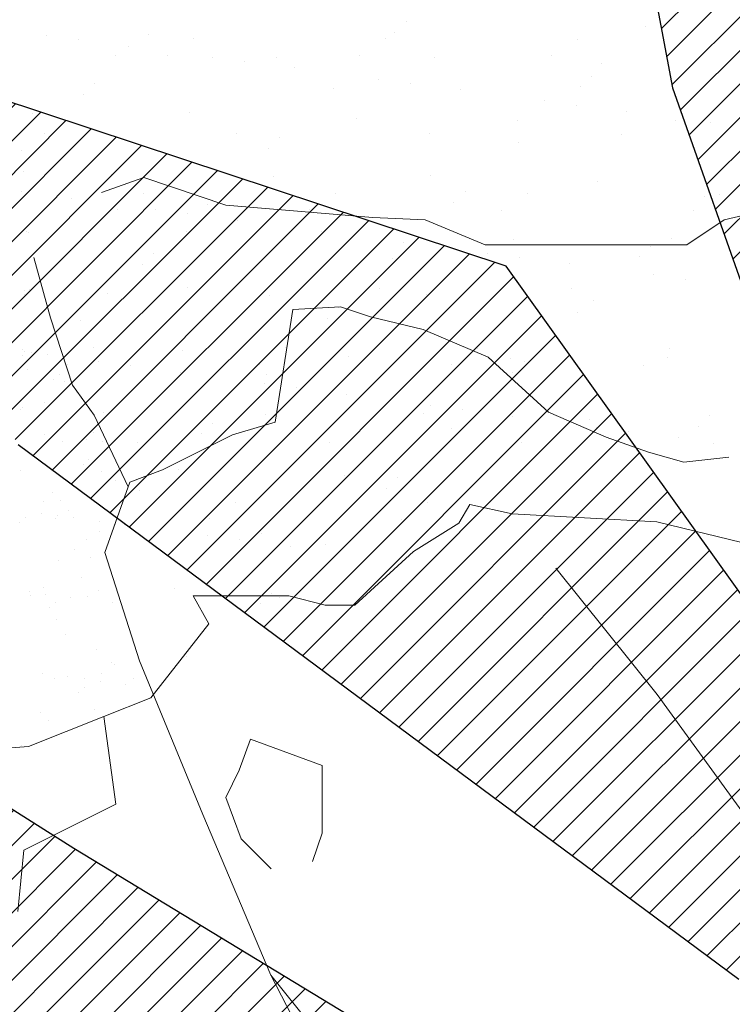
# Model space of a CAD drawing. Units: inches. Extents: x 1986 to 21484, y -1816 to 2016.
# Tile 23 of 85: x 2162.297 to 2166.915, y 1891.95 to 1898.331. Entities that reach past the tile are written whole.
import ezdxf

# ---------------------------------------------------------------- set-up
doc = ezdxf.new("R2010")
doc.units = ezdxf.units.IN
doc.layers.add('L-PLNT', color=84, linetype='Continuous', lineweight=13)
doc.layers.add('vfolhas', color=114, linetype='Continuous', lineweight=5)
doc.layers.add('vfolha2', color=110, linetype='Continuous')
doc.layers.add('vfolhas2', color=102, linetype='Continuous')
pattern_1 = [(45, (-2446.5133113, 50.986076), (-0.004419417382, 0.004419417382), [])]

# ---------------------------------------------------------------- blocks, each defined once
blk = doc.blocks.new('arbusto_PB_verde_grande')
at = {"layer": 'vfolha2'}
h = blk.add_hatch(dxfattribs=at)
h.set_pattern_fill('ANSI31', color=256, scale=0.05, style=0)
h.set_pattern_definition(pattern_1)
h.paths.add_polyline_path([(-0.18963, 0.29704), (-0.08553, 0.20192), (-0.10785, 0.25007), (-0.13202, 0.31865), (-0.25096, 0.48479), (-0.44952, 0.5505), (-0.37946, 0.43789)])
h.paths.add_polyline_path([(0.07911, -0.4071), (0.08214, -0.50631), (0.17255, -0.6355), (0.18428, -0.44151), (0.14904, -0.29177), (0.02625, -0.03934), (0.03527, -0.25376)])
at = {"layer": 'vfolhas'}
h = blk.add_hatch(dxfattribs=at)
h.set_pattern_fill('ANSI31', color=256, scale=0.05, style=0)
h.set_pattern_definition(pattern_1)
h.paths.add_polyline_path([(-0.07279, 0.50669), (-0.18085, 0.65063), (-0.2334, 0.67253), (-0.20712, 0.53176), (-0.10785, 0.25007), (0.02625, -0.03934), (0.00028, 0.09048), (0.00816, 0.16241), (-0.04939, 0.29079)])
h.paths.add_polyline_path([(0.09902, 0.41929), (0.09372, 0.26573), (0.07906, 0.18814), (0.15506, 0.36901), (0.26606, 0.5505), (0.28356, 0.63504), (0.2485, 0.68819), (0.25145, 0.63504), (0.20178, 0.54426)])
h.paths.add_polyline_path([(0.12295, 0.24073), (0.047, 0.06233), (0.02625, -0.03934), (0.11122, 0.04358), (0.18428, 0.09364), (0.27478, 0.19376), (0.3215, 0.25323), (0.44129, 0.38467), (0.47634, 0.57866), (0.41789, 0.45347), (0.28939, 0.30954)])
h.paths.add_polyline_path([(0.58145, -0.03779), (0.70707, 0.01536), (0.78591, 0.04667), (0.74796, 0.06549), (0.62818, 0.08423), (0.52595, 0.09048), (0.39745, 0.04358), (0.02625, -0.03934), (0.25728, -0.03154), (0.43834, -0.0347)])
h.paths.add_polyline_path([(0.52022, -0.03647), (0.43834, -0.0347), (0.25728, -0.03154), (0.02625, -0.03934), (0.17964, -0.08515), (0.53768, -0.13167), (0.69541, -0.15357), (0.78591, -0.07852), (0.70413, -0.10042)])
h.paths.add_polyline_path([(0.27189, -0.21929), (0.14922, -0.14107), (0.02625, -0.03934), (0.15794, -0.31007), (0.29522, -0.42585), (0.41789, -0.49157), (0.56396, -0.56669), (0.5114, -0.48532), (0.39456, -0.34139)])
h.paths.add_polyline_path([(-0.05818, -0.47591), (-0.02312, -0.61984), (0.047, -0.80134), (0.08494, -0.59794), (0.07911, -0.4071), (0.03527, -0.25376), (0.02625, -0.03934), (-0.03773, -0.26001)])
h.paths.add_polyline_path([(-0.24218, 0.14054), (-0.11073, 0.06858), (0.02625, -0.03934), (-0.04235, 0.10871), (-0.21007, 0.23757), (-0.36485, 0.33145), (-0.47874, 0.40341), (-0.54303, 0.46288), (-0.49041, 0.33145), (-0.39408, 0.22192)])
at = {"layer": 'vfolha2'}
for p, q in [((-0.25096, 0.48479), (-0.44952, 0.5505)), ((-0.13202, 0.31865), (-0.25096, 0.48479)), ((-0.37946, 0.43789), (-0.18963, 0.29704))]:
    blk.add_line(p, q, dxfattribs=at)
at = {"layer": 'vfolhas2'}
for p, q in [((-0.2334, 0.67253), (-0.20712, 0.53176)), ((-0.20712, 0.53176), (-0.10785, 0.25007)), ((-0.36485, 0.33145), (-0.47874, 0.40341)), ((-0.21007, 0.23757), (-0.36485, 0.33145))]:
    blk.add_line(p, q, dxfattribs=at)
blk = doc.blocks.new('PLANT-SHRUB')
for p, q in [((2164.8017, 1898.3163), (2164.8017, 1898.3163)), ((2162.47, 1898.2297), (2162.47, 1898.2297)), ((2163.1287, 1898.235), (2163.1287, 1898.235)), ((2164.728, 1898.2488), (2164.728, 1898.2488)), ((2166.3509, 1898.2841), (2166.3509, 1898.2841)), ((2162.678, 1898.2023), (2162.678, 1898.2023)), ((2163.0029, 1898.1596), (2163.0029, 1898.1596)), ((2163.421, 1898.2083), (2163.421, 1898.2083)), ((2164.6656, 1898.206), (2164.6656, 1898.206)), ((2165.9103, 1898.2038), (2165.9103, 1898.2038)), ((2162.9177, 1898.0971), (2162.9177, 1898.0971)), ((2163.2525, 1898.1009), (2163.2525, 1898.1009)), ((2164.4971, 1898.0987), (2164.4971, 1898.0987)), ((2165.7417, 1898.0964), (2165.7417, 1898.0964)), ((2163.5458, 1898.0881), (2163.5458, 1898.0881)), ((2163.7538, 1898.0607), (2163.7538, 1898.0607)), ((2163.9638, 1898.0837), (2163.9638, 1898.0837)), ((2164.9862, 1898.0886), (2164.9862, 1898.0886)), ((2166.0657, 1898.0497), (2166.0657, 1898.0497)), ((2164.0787, 1898.0179), (2164.0787, 1898.0179)), ((2162.781, 1897.9164), (2162.781, 1897.9164)), ((2164.6216, 1897.9464), (2164.6216, 1897.9464)), ((2164.8296, 1897.9191), (2164.8296, 1897.9191)), ((2166.0031, 1897.9655), (2166.0031, 1897.9655)), ((2162.7074, 1897.8489), (2162.7074, 1897.8489)), ((2164.3302, 1897.8842), (2164.3302, 1897.8842)), ((2165.1546, 1897.8763), (2165.1546, 1897.8763)), ((2165.9295, 1897.898), (2165.9295, 1897.898)), ((2165.6974, 1897.8048), (2165.6974, 1897.8048)), ((2165.9055, 1897.7774), (2165.9055, 1897.7774)), ((2162.3772, 1897.7223), (2162.3772, 1897.7223)), ((2163.3996, 1897.7273), (2163.3996, 1897.7273)), ((2166.2304, 1897.7346), (2166.2304, 1897.7346)), ((2164.4791, 1897.6884), (2164.4791, 1897.6884)), ((2165.5253, 1897.675), (2165.5253, 1897.675)), ((2166.5477, 1897.6799), (2166.5477, 1897.6799)), ((2166.7733, 1897.6632), (2166.7733, 1897.6632)), ((2162.4603, 1897.5963), (2162.4603, 1897.5963)), ((2163.705, 1897.594), (2163.705, 1897.594)), ((2164.9496, 1897.5918), (2164.9496, 1897.5918)), ((2166.1942, 1897.5895), (2166.1942, 1897.5895)), ((2163.9825, 1897.5656), (2163.9825, 1897.5656)), ((2165.5317, 1897.5335), (2165.5317, 1897.5335)), ((2162.3096, 1897.4844), (2162.3096, 1897.4844)), ((2162.3096, 1897.4844), (2162.3096, 1897.4844)), ((2163.9088, 1897.4981), (2163.9088, 1897.4981)), ((2162.3185, 1897.3493), (2162.3185, 1897.3493)), ((2163.1007, 1897.3074), (2162.8262, 1897.2106)), ((2162.8925, 1897.327), (2162.8925, 1897.327)), ((2163.6336, 1897.1299), (2163.1007, 1897.3074)), ((2163.9387, 1897.3136), (2163.9387, 1897.3136)), ((2164.9611, 1897.3185), (2164.9611, 1897.3185)), ((2166.0405, 1897.2796), (2166.0405, 1897.2796)), ((2162.3095, 1897.216), (2162.3095, 1897.216)), ((2162.3095, 1897.216), (2162.3095, 1897.216)), ((2162.3095, 1897.216), (2162.3095, 1897.216)), ((2163.0982, 1897.2075), (2163.0982, 1897.2075)), ((2164.3428, 1897.2052), (2164.3428, 1897.2052)), ((2165.184, 1897.2148), (2165.184, 1897.2148)), ((2165.5875, 1897.203), (2165.5875, 1897.203)), ((2166.8321, 1897.2007), (2166.8321, 1897.2007)), ((2162.6344, 1897.1733), (2162.6344, 1897.1733)), ((2165.1103, 1897.1473), (2165.1103, 1897.1473)), ((2166.7331, 1897.1827), (2166.7331, 1897.1827)), ((2162.9297, 1897.1001), (2162.9297, 1897.1001)), ((2163.1773, 1897.1018), (2163.1773, 1897.1018)), ((2163.3853, 1897.0744), (2163.3853, 1897.0744)), ((2163.511, 1897.1336), (2163.511, 1897.1336)), ((2164.5862, 1897.0492), (2163.6336, 1897.1299)), ((2164.1743, 1897.0979), (2164.1743, 1897.0979)), ((2165.4189, 1897.0956), (2165.4189, 1897.0956)), ((2166.6636, 1897.0933), (2166.6636, 1897.0933)), ((2167.202, 1897.1138), (2166.8629, 1897.0331)), ((2163.7102, 1897.0316), (2163.7102, 1897.0316)), ((2164.9253, 1897.0331), (2164.5862, 1897.0492)), ((2165.3128, 1896.8718), (2164.9253, 1897.0331)), ((2166.8629, 1897.0331), (2166.6207, 1896.8718)), ((2162.3402, 1896.9614), (2162.3402, 1896.9614)), ((2162.3521, 1896.9523), (2162.3521, 1896.9523)), ((2162.3521, 1896.9523), (2162.3521, 1896.9523)), ((2163.3745, 1896.9572), (2163.3745, 1896.9572)), ((2164.2531, 1896.9602), (2164.2531, 1896.9602)), ((2164.4539, 1896.9183), (2164.4539, 1896.9183)), ((2164.4611, 1896.9328), (2164.4611, 1896.9328)), ((2164.7861, 1896.89), (2164.7861, 1896.89)), ((2165.5001, 1896.9049), (2165.5001, 1896.9049)), ((2166.5225, 1896.9098), (2166.5225, 1896.9098)), ((2165.3128, 1896.8718), (2165.3128, 1896.8718)), ((2165.8457, 1896.8718), (2165.3128, 1896.8718)), ((2165.3289, 1896.8185), (2165.3289, 1896.8185)), ((2166.2655, 1896.8718), (2165.8457, 1896.8718)), ((2166.6207, 1896.8718), (2166.2655, 1896.8718)), ((2166.3854, 1896.8641), (2166.3854, 1896.8641)), ((2162.4964, 1896.3984), (2162.3874, 1896.7903)), ((2163.1633, 1896.815), (2163.1633, 1896.815)), ((2164.7125, 1896.7828), (2164.7125, 1896.7828)), ((2165.537, 1896.7911), (2165.537, 1896.7911)), ((2166.3118, 1896.7966), (2166.3118, 1896.7966)), ((2163.0897, 1896.7475), (2163.0897, 1896.7475)), ((2165.8619, 1896.7484), (2165.8619, 1896.7484)), ((2166.4048, 1896.6769), (2166.4048, 1896.6769)), ((2166.6128, 1896.6495), (2166.6128, 1896.6495)), ((2162.3276, 1896.5763), (2162.3276, 1896.5763)), ((2162.362, 1896.5813), (2162.362, 1896.5813)), ((2162.3918, 1896.6008), (2162.3918, 1896.6008)), ((2163.3822, 1896.5932), (2163.3822, 1896.5932)), ((2164.6268, 1896.5909), (2164.6268, 1896.5909)), ((2165.8714, 1896.5887), (2165.8714, 1896.5887)), ((2162.3251, 1896.5476), (2162.3251, 1896.5476)), ((2162.8673, 1896.5569), (2162.8673, 1896.5569)), ((2163.9135, 1896.5435), (2163.9135, 1896.5435)), ((2164.9359, 1896.5484), (2164.9359, 1896.5484)), ((2166.0154, 1896.5096), (2166.0154, 1896.5096)), ((2163.9528, 1895.7227), (2164.0665, 1896.4531)), ((2164.0665, 1896.4531), (2164.3751, 1896.4694)), ((2164.0665, 1896.4531), (2164.0665, 1896.4531)), ((2164.3648, 1896.4642), (2164.3648, 1896.4642)), ((2164.3751, 1896.4694), (2164.5701, 1896.4044)), ((2164.3751, 1896.4694), (2164.3751, 1896.4694)), ((2162.638, 1895.9629), (2162.4964, 1896.3984)), ((2162.6919, 1896.383), (2162.6919, 1896.383)), ((2164.2911, 1896.3967), (2164.2911, 1896.3967)), ((2164.5701, 1896.4044), (2164.9112, 1896.3233)), ((2165.914, 1896.432), (2165.914, 1896.432)), ((2164.9112, 1896.3233), (2165.3335, 1896.1447)), ((2162.315, 1896.1913), (2162.315, 1896.1913)), ((2162.3269, 1896.1822), (2162.3269, 1896.1822)), ((2162.3269, 1896.1822), (2162.3269, 1896.1822)), ((2162.7754, 1896.2067), (2162.7754, 1896.2067)), ((2163.3493, 1896.1871), (2163.3493, 1896.1871)), ((2164.0201, 1896.2044), (2164.0201, 1896.2044)), ((2165.2647, 1896.2022), (2165.2647, 1896.2022)), ((2166.5093, 1896.1999), (2166.5093, 1896.1999)), ((2162.3146, 1896.1541), (2162.3146, 1896.1541)), ((2162.3749, 1896.1726), (2162.3749, 1896.1726)), ((2162.4789, 1896.1589), (2162.4789, 1896.1589)), ((2164.4287, 1896.1482), (2164.4287, 1896.1482)), ((2165.3335, 1896.1447), (2165.7234, 1895.7876)), ((2165.3335, 1896.1447), (2165.3335, 1896.1447)), ((2165.4749, 1896.1348), (2165.4749, 1896.1348)), ((2166.4973, 1896.1397), (2166.4973, 1896.1397)), ((2162.3441, 1896.0644), (2162.3441, 1896.0644)), ((2162.3441, 1896.0644), (2162.3441, 1896.0644)), ((2162.6069, 1896.0993), (2162.6069, 1896.0993)), ((2162.8088, 1896.1155), (2162.8088, 1896.1155)), ((2163.0168, 1896.0881), (2163.0168, 1896.0881)), ((2163.8515, 1896.097), (2163.8515, 1896.097)), ((2165.0962, 1896.0948), (2165.0962, 1896.0948)), ((2165.5662, 1896.1134), (2165.5662, 1896.1134)), ((2166.3408, 1896.0925), (2166.3408, 1896.0925)), ((2162.5163, 1895.9968), (2162.5163, 1895.9968)), ((2162.5531, 1896.0306), (2162.5531, 1896.0306)), ((2163.3417, 1896.0453), (2163.3417, 1896.0453)), ((2163.8933, 1896.0322), (2163.8933, 1896.0322)), ((2165.4926, 1896.0459), (2165.4926, 1896.0459)), ((2162.5845, 1895.9845), (2162.5845, 1895.9845)), ((2162.7797, 1895.7669), (2162.638, 1895.9629)), ((2163.8846, 1895.9739), (2163.8846, 1895.9739)), ((2164.0926, 1895.9465), (2164.0926, 1895.9465)), ((2164.4176, 1895.9037), (2164.4176, 1895.9037)), ((2162.3024, 1895.8062), (2162.3024, 1895.8062)), ((2162.3174, 1895.8146), (2162.3174, 1895.8146)), ((2162.4566, 1895.847), (2162.4566, 1895.847)), ((2164.9604, 1895.8322), (2164.9604, 1895.8322)), ((2165.1685, 1895.8048), (2165.1685, 1895.8048)), ((2162.9997, 1895.3027), (2162.7797, 1895.7669)), ((2162.8421, 1895.7868), (2162.8421, 1895.7868)), ((2163.8883, 1895.7734), (2163.8883, 1895.7734)), ((2164.9107, 1895.7783), (2164.9107, 1895.7783)), ((2165.4934, 1895.7621), (2165.4934, 1895.7621)), ((2165.7234, 1895.7876), (2166.097, 1895.6253)), ((2165.7234, 1895.7876), (2165.7234, 1895.7876)), ((2165.9902, 1895.7395), (2165.9902, 1895.7395)), ((2166.7677, 1895.7626), (2166.7677, 1895.7626)), ((2163.5456, 1895.7136), (2163.5456, 1895.7136)), ((2163.6766, 1895.6415), (2163.9528, 1895.7227)), ((2165.0948, 1895.6814), (2165.0948, 1895.6814)), ((2166.0363, 1895.6906), (2166.0363, 1895.6906)), ((2166.694, 1895.6951), (2166.694, 1895.6951)), ((2162.4571, 1895.6444), (2162.4571, 1895.6444)), ((2162.7286, 1895.6086), (2162.7286, 1895.6086)), ((2162.7756, 1895.6526), (2162.7756, 1895.6526)), ((2163.2218, 1895.4143), (2163.6766, 1895.6415)), ((2163.4719, 1895.6461), (2163.4719, 1895.6461)), ((2166.097, 1895.6253), (2166.3732, 1895.5279)), ((2166.2443, 1895.6632), (2166.2443, 1895.6632)), ((2166.5692, 1895.6204), (2166.5692, 1895.6204)), ((2162.5719, 1895.5994), (2162.5719, 1895.5994)), ((2162.6913, 1895.5989), (2162.6913, 1895.5989)), ((2162.8326, 1895.595), (2162.8326, 1895.595)), ((2163.0594, 1895.5924), (2163.0594, 1895.5924)), ((2164.304, 1895.5901), (2164.304, 1895.5901)), ((2165.5486, 1895.5879), (2165.5486, 1895.5879)), ((2166.7933, 1895.5856), (2166.7933, 1895.5856)), ((2162.7443, 1895.4799), (2162.7443, 1895.4799)), ((2166.3732, 1895.5279), (2166.6006, 1895.463)), ((2166.6006, 1895.463), (2166.893, 1895.4955)), ((2166.893, 1895.4955), (2166.893, 1895.4955)), ((2162.7074, 1895.4461), (2162.7074, 1895.4461)), ((2163.0106, 1895.3331), (2163.2218, 1895.4143)), ((2163.3241, 1895.417), (2163.3241, 1895.417)), ((2162.3017, 1895.4121), (2162.3017, 1895.4121)), ((2162.3017, 1895.4121), (2162.3017, 1895.4121)), ((2162.8295, 1895.4017), (2162.8295, 1895.4017)), ((2164.4036, 1895.3781), (2164.4036, 1895.3781)), ((2164.7471, 1895.3628), (2164.7471, 1895.3628)), ((2162.8481, 1894.8786), (2163.0106, 1895.3331)), ((2162.8481, 1894.8786), (2162.9997, 1895.3027)), ((2162.9175, 1895.3454), (2162.9175, 1895.3454)), ((2164.6734, 1895.2953), (2164.6734, 1895.2953)), ((2162.5085, 1895.2639), (2162.5085, 1895.2639)), ((2163.0741, 1895.2815), (2163.0741, 1895.2815)), ((2162.4526, 1895.2059), (2162.4526, 1895.2059)), ((2162.4526, 1895.2059), (2162.4526, 1895.2059)), ((2162.5593, 1895.2144), (2162.5593, 1895.2144)), ((2163.6973, 1895.2036), (2163.6973, 1895.2036)), ((2164.9419, 1895.2013), (2164.9419, 1895.2013)), ((2165.1435, 1895.0672), (2165.2147, 1895.1892)), ((2165.2147, 1895.1892), (2165.4893, 1895.1282)), ((2162.3347, 1895.1046), (2162.3347, 1895.1046)), ((2162.4403, 1895.1292), (2162.4403, 1895.1292)), ((2162.4403, 1895.1292), (2162.4403, 1895.1292)), ((2162.5299, 1895.0985), (2162.5299, 1895.0985)), ((2162.5443, 1895.1155), (2162.5443, 1895.1155)), ((2162.6142, 1895.1522), (2162.6142, 1895.1522)), ((2162.6483, 1895.1018), (2162.6483, 1895.1018)), ((2162.6483, 1895.1018), (2162.6483, 1895.1018)), ((2162.6483, 1895.1018), (2162.6483, 1895.1018)), ((2163.5287, 1895.0962), (2163.5287, 1895.0962)), ((2165.4893, 1895.1282), (2166.4251, 1895.0774)), ((2162.2978, 1895.0708), (2162.2978, 1895.0708)), ((2162.8108, 1895.0804), (2162.8108, 1895.0804)), ((2162.9733, 1895.059), (2162.9733, 1895.059)), ((2164.7734, 1895.094), (2164.7734, 1895.094)), ((2164.8485, 1894.8843), (2165.1435, 1895.0672)), ((2166.4251, 1895.0774), (2167.1371, 1894.9046)), ((2162.817, 1895.0167), (2162.817, 1895.0167)), ((2162.817, 1895.0167), (2162.817, 1895.0167)), ((2162.817, 1895.0167), (2162.817, 1895.0167)), ((2163.5161, 1894.9876), (2163.5161, 1894.9876)), ((2163.8631, 1895.0033), (2163.8631, 1895.0033)), ((2162.7264, 1894.9629), (2162.7264, 1894.9629)), ((2162.7264, 1894.9629), (2162.7264, 1894.9629)), ((2163.7242, 1894.9602), (2163.7242, 1894.9602)), ((2164.0491, 1894.9174), (2164.0491, 1894.9174)), ((2164.2756, 1894.9308), (2164.2756, 1894.9308)), ((2162.6528, 1894.8954), (2162.6528, 1894.8954)), ((2162.6528, 1894.8954), (2162.6528, 1894.8954)), ((2162.7561, 1894.845), (2162.7561, 1894.845)), ((2163.0739, 1894.1758), (2162.8481, 1894.8786)), ((2164.4688, 1894.5366), (2164.8485, 1894.8843)), ((2164.8485, 1894.8843), (2164.8485, 1894.8843)), ((2162.5467, 1894.8293), (2162.5467, 1894.8293)), ((2162.6997, 1894.7132), (2162.6997, 1894.7132)), ((2166.4276, 1893.9579), (2165.771, 1894.7754)), ((2162.4528, 1894.6518), (2162.4528, 1894.6518)), ((2162.3601, 1894.6224), (2162.3601, 1894.6224)), ((2162.3685, 1894.5981), (2162.3685, 1894.5981)), ((2162.4641, 1894.6087), (2162.4641, 1894.6087)), ((2162.6265, 1894.5873), (2162.6265, 1894.5873)), ((2162.7366, 1894.5916), (2162.7366, 1894.5916)), ((2162.7366, 1894.5916), (2162.7366, 1894.5916)), ((2162.8044, 1894.6316), (2162.8044, 1894.6316)), ((2163.2989, 1894.6469), (2163.2989, 1894.6469)), ((2163.4212, 1894.5976), (2164.0416, 1894.5976)), ((2163.4212, 1894.5976), (2163.4212, 1894.5976)), ((2163.5229, 1894.4146), (2163.4212, 1894.5976)), ((2163.9279, 1894.6122), (2163.9279, 1894.6122)), ((2163.9812, 1894.5893), (2163.9812, 1894.5893)), ((2164.0416, 1894.5976), (2164.2756, 1894.5366)), ((2162.5258, 1894.5539), (2162.5258, 1894.5539)), ((2162.898, 1894.5515), (2162.898, 1894.5515)), ((2163.8542, 1894.5446), (2163.8542, 1894.5446)), ((2164.2756, 1894.5366), (2164.4688, 1894.5366)), ((2162.489, 1894.5201), (2162.489, 1894.5201)), ((2162.5342, 1894.4443), (2162.5342, 1894.4443)), ((2163.1465, 1893.9369), (2163.5229, 1894.4146)), ((2162.5948, 1894.3446), (2162.5948, 1894.3446)), ((2162.7918, 1894.2466), (2162.7918, 1894.2466)), ((2162.7918, 1894.2466), (2162.7918, 1894.2466)), ((2162.7918, 1894.2466), (2162.7918, 1894.2466)), ((2163.3745, 1894.2028), (2163.3745, 1894.2028)), ((2162.8908, 1894.1625), (2162.8908, 1894.1625)), ((2162.9137, 1894.1502), (2162.9137, 1894.1502)), ((2163.4826, 1893.1809), (2163.0739, 1894.1758)), ((2162.4423, 1894.0941), (2162.4423, 1894.0941)), ((2162.8294, 1894.0965), (2162.8294, 1894.0965)), ((2162.5216, 1894.0592), (2162.5216, 1894.0592)), ((2162.6048, 1894.0727), (2162.6048, 1894.0727)), ((2162.6048, 1894.0727), (2162.6048, 1894.0727)), ((2162.7137, 1894.0584), (2162.7137, 1894.0584)), ((2162.8177, 1894.0447), (2162.8177, 1894.0447)), ((2162.9802, 1894.0233), (2162.9802, 1894.0233)), ((2163.0328, 1894.0617), (2163.0328, 1894.0617)), ((2162.6801, 1893.9694), (2162.6801, 1893.9694)), ((2162.7169, 1894.0032), (2162.7169, 1894.0032)), ((2167.1381, 1892.979), (2166.4276, 1893.9579)), ((2162.8414, 1893.815), (2163.1465, 1893.9369)), ((2162.4334, 1893.8442), (2162.4334, 1893.8442)), ((2162.7792, 1893.8615), (2162.7792, 1893.8615)), ((2162.3532, 1893.6218), (2162.8414, 1893.815)), ((2162.4812, 1893.7871), (2162.4812, 1893.7871)), ((2162.8414, 1893.815), (2162.92, 1893.2475)), ((2162.8414, 1893.815), (2162.8414, 1893.815)), ((2162.3074, 1893.6278), (2162.3074, 1893.6278)), ((2163.7921, 1893.669), (2163.7182, 1893.4682)), ((2164.2561, 1893.4981), (2163.7921, 1893.669)), ((2162.2413, 1893.6117), (2162.3532, 1893.6218)), ((2163.7182, 1893.4682), (2163.6333, 1893.2907)), ((2164.2561, 1893.4981), (2164.2561, 1893.4981)), ((2164.2561, 1893.0589), (2164.2561, 1893.4981)), ((2162.92, 1893.2475), (2162.3233, 1892.9494)), ((2163.6333, 1893.2907), (2163.731, 1893.0222)), ((2163.9242, 1892.1391), (2163.4826, 1893.1809)), ((2164.1951, 1892.8758), (2164.2561, 1893.0589)), ((2163.731, 1893.0222), (2163.9264, 1892.827)), ((2162.3233, 1892.9494), (2162.2835, 1892.5519)), ((2163.9242, 1892.1391), (2164.3896, 1891.5609)), ((2164.5252, 1890.9746), (2163.9242, 1892.1391))]:
    blk.add_line(p, q)

msp = doc.modelspace()

# ---------------------------------------------------------------- block references
at = {"layer": 'L-PLNT'}
msp.add_blockref('PLANT-SHRUB', (0, 0), dxfattribs=at)
at = {"layer": 'L-PLNT', "xscale": 24.60366729364114, "yscale": 24.60366729364114, "zscale": 24.60366729364114}
msp.add_blockref('arbusto_PB_verde_grande', (2171.6234, 1884.8051), dxfattribs=at)

doc.saveas('drawing.dxf')
